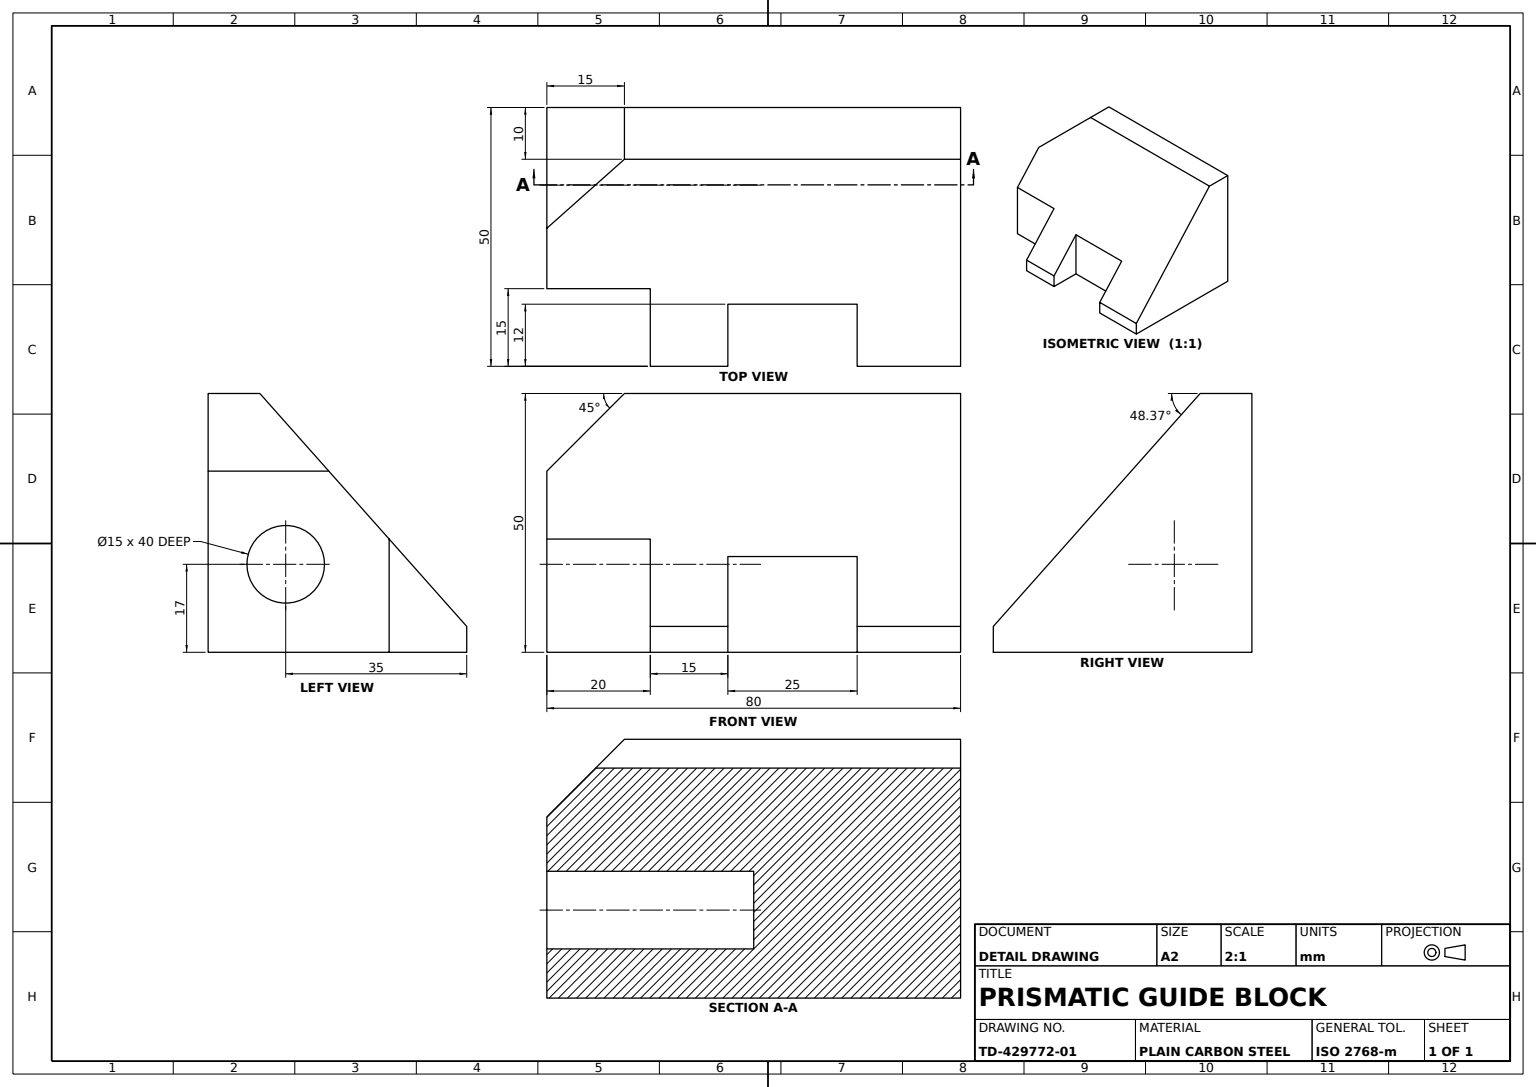
from build123d import *

# Parameters (mm, degrees)
BRACKET_BODY_DEPTH          = 80
BASE_NOTCH_SKETCH_W         = 15
BASE_NOTCH_SKETCH_H         = 20
BASE_NOTCH_SKETCH_W_2       = 12
BASE_NOTCH_SKETCH_H_2       = 25
BASE_NOTCH_CUT_DEPTH        = 80
SIDE_HOLE_SKETCH_R          = 7.5
SIDE_HOLE_DEPTH             = 40
HALF_LENGTH_BEVEL_CUT_DEPTH = 40


with BuildPart() as part:
    # Bracket Profile Sketch → Bracket Body (new body)
    with BuildSketch(Plane.XY):
        Polygon((0, 0), (50, 0), (50, 5), (10, 50), (0, 50), align=None)
    extrude(amount=BRACKET_BODY_DEPTH)

    # Base Notch Sketch → Base Notch Cut (cut)
    with BuildSketch(Plane.XZ):
        with Locations((42.5, 70)):
            Rectangle(BASE_NOTCH_SKETCH_W, BASE_NOTCH_SKETCH_H)
        with Locations((44, 32.5)):
            Rectangle(BASE_NOTCH_SKETCH_W_2, BASE_NOTCH_SKETCH_H_2)
    extrude(amount=-BASE_NOTCH_CUT_DEPTH, mode=Mode.SUBTRACT)

    # Side Hole Sketch → Side Hole (cut)
    with BuildSketch(Plane.XY.offset(80)):
        with Locations((15, 17)):
            Circle(SIDE_HOLE_SKETCH_R)
    extrude(amount=-SIDE_HOLE_DEPTH, mode=Mode.SUBTRACT)

    # Half-Length Bevel Sketch → Half-Length Bevel Cut (cut)
    with BuildSketch(Plane.ZY):
        Polygon((80, 35), (65, 50), (80, 50), align=None)
    extrude(amount=-HALF_LENGTH_BEVEL_CUT_DEPTH, mode=Mode.SUBTRACT)


solid = part.part
